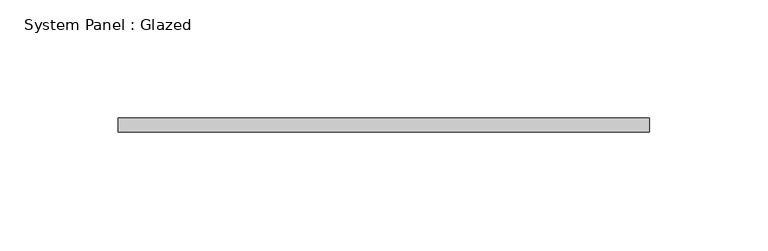
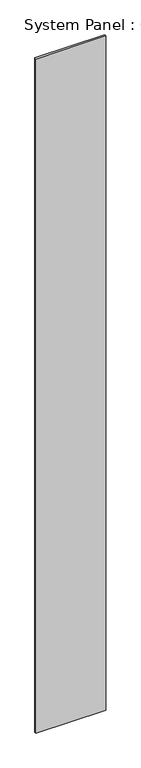
"""IFC4 building model written with IfcOpenShell, lengths in millimetres: plate geometry, System Panel : Glazed."""

from ifc_helpers import new_model, si_unit, origin, origin_with_axes, place, context, project, spatial, polyline, outline, extrude, source, transform, mapped, element, save


def system_panel_glazed_6a0df73a(model_context):
    return source(origin(), model_context, "Body", "SweptSolid", [
        extrude(outline(polyline([(112.5, 34.0), (-112.5, 34.0), (-112.5, 40.0), (112.5, 40.0), (112.5, 34.0)])), origin_with_axes(), (0.0, 0.0, 1.0), 2300.0),
    ])


if __name__ == "__main__":
    model = new_model("IFC4")
    model_context = context("Model", 3, world=origin())
    ifc_project = project(units=[si_unit("LENGTHUNIT", "METRE", prefix="MILLI")], contexts=[model_context])
    site = spatial("IfcSite", under=ifc_project)
    building = spatial("IfcBuilding", under=site)
    placement = place(None, origin())
    system_panel_glazed_shape = system_panel_glazed_6a0df73a(model_context)
    element("IfcPlate", 1, ObjectType="System Panel : Glazed", at=placement, inside=building, context=model_context, shape_type="MappedRepresentation", body=[
        mapped(system_panel_glazed_shape, transform((0.0, 0.0, 0.0), x_axis=(1.0, 0.0, 0.0), y_axis=(0.0, 1.0, 0.0), z_axis=(0.0, 0.0, 1.0))),
    ])
    save(model, "model.ifc")

# Revit data of these elements
# Type "System Panel : Glazed"
#   Construction Type Id = "GSP4R"
#   Analytic Construction = "1/8 in Pilkington single glazing"
#   Visual Light Transmittance = 0.9
#   Solar Heat Gain Coefficient = 0.86
#   Heat Transfer Coefficient (U) = 6.7069 W/(m²·K)
#   Define Thermal Properties by = 1
# Element 1 (IfcPlate, "System Panel : Glazed")
#   Materials on its faces: "Default New Material(6)"
# Materials
#   "Default New Material(6)": class "Generic", colour RGB 191 25 25, transparency 0.9, Cost = 0
